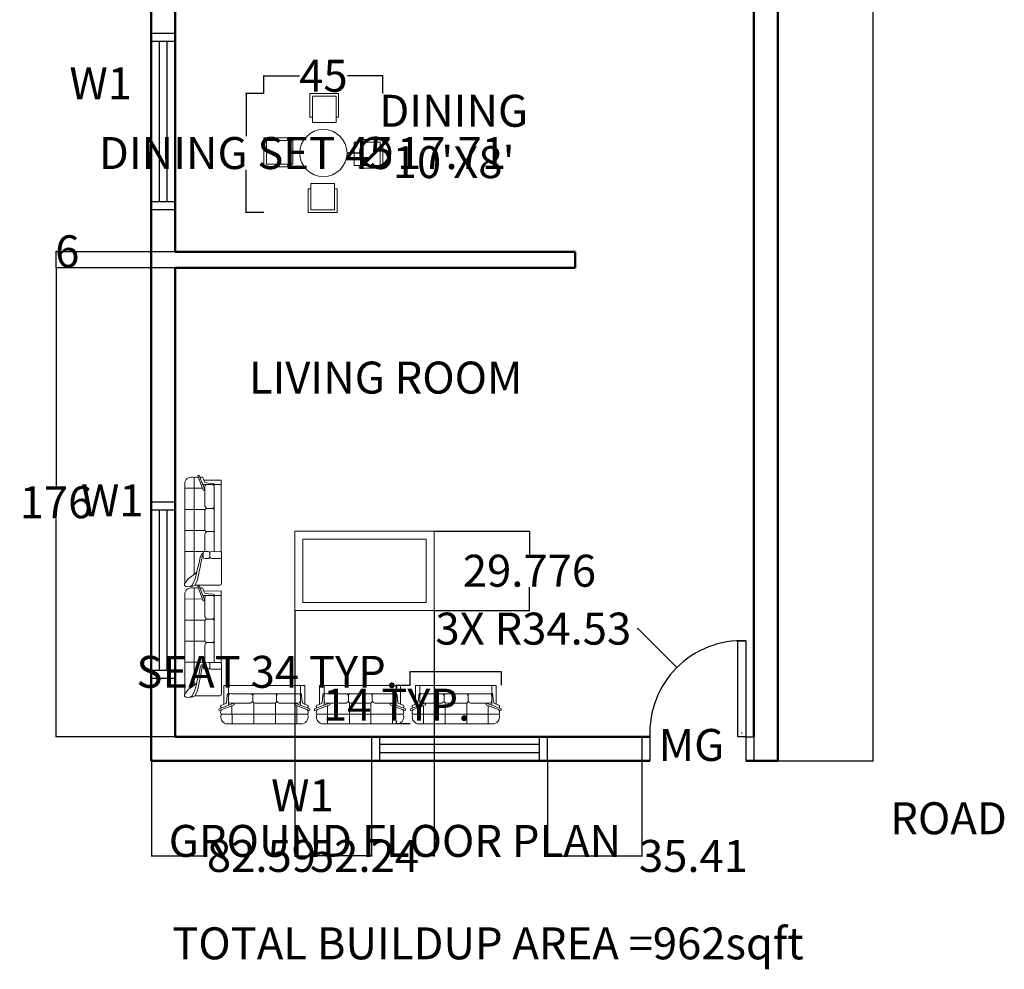
# Model space of a CAD drawing. Units: inches. Extents: x -15 to 810, y -55 to 662.
# Tile 1 of 3: x -7 to 362, y -55 to 302. Entities that reach past the tile are written whole.
import ezdxf
from ezdxf.enums import TextEntityAlignment as Align

# ---------------------------------------------------------------- set-up
doc = ezdxf.new("R2010")
doc.units = ezdxf.units.IN
doc.header["$MEASUREMENT"] = 0
for name, color, linetype, lineweight in [('A-ANNO-DIMS', 2, 'Continuous', 18), ('A-ANNO-TEXT', 1, 'Continuous', 25), ('A-AREA-IDEN', 1, 'Continuous', 25), ('A-DOOR', 2, 'Continuous', 25), ('A-FURN', 8, 'Continuous', 18), ('A-GLAZ', 4, 'Continuous', 18), ('A-WALL', 6, 'Continuous', 50)]:
    doc.layers.add(name, color=color, linetype=linetype, lineweight=lineweight)
doc.layers.add('Layer3', color=4, linetype='Continuous')
doc.styles.get("Standard").update_dxf_attribs({"font": 'arial.ttf'})
doc.dimstyles.get("Standard").update_dxf_attribs({"dimtxt": 12, "dimasz": 0.18, "dimexe": 0.18, "dimexo": 0.0625, "dimgap": 0.09, "dimtad": 0, "dimtih": 1, "dimtoh": 1, "dimdec": 0, "dimzin": 0, "dimdsep": 46, "dimlunit": 4, "dimtxsty": 'Standard', "dimcen": 0.09, "dimadec": 0, "dimazin": 0, "dimtfac": 1, "dimtdec": 0, "dimtofl": 0, "dimtmove": 0, "dimatfit": 3, "dimfxl": 1, "dimtolj": 1, "dimtzin": 0, "dimarcsym": 0})

# ---------------------------------------------------------------- blocks, each defined once
blk = doc.blocks.new('A$C21DD57CF')
for p, q in [((0, 682), (8, 763)), ((0, 682), (8, 763)), ((37, 628), (0, 682)), ((37, 628), (0, 682)), ((8, 763), (29, 794)), ((8, 763), (29, 794)), ((16, 616), (16, 655)), ((16, 616), (16, 655)), ((29, 794), (63, 792)), ((29, 794), (63, 792)), ((63, 792), (74, 786)), ((63, 792), (74, 786)), ((74, 786), (2250, 786)), ((74, 786), (173, 714)), ((74, 786), (2250, 786)), ((74, 786), (173, 714)), ((173, 714), (247, 611)), ((173, 714), (247, 611)), ((640, 786), (761, 786)), ((640, 786), (761, 786)), ((761, 786), (761, 356)), ((761, 786), (761, 356)), ((1211, 356), (1211, 786)), ((1211, 786), (1661, 786)), ((1211, 356), (1211, 786)), ((1211, 786), (1661, 786)), ((1661, 786), (1661, 347)), ((1661, 786), (1661, 347)), ((2116, 783), (2119, 410)), ((2116, 783), (2119, 410)), ((35, 572), (16, 616)), ((35, 572), (16, 616)), ((35, 574), (141, 516)), ((35, 574), (141, 516)), ((36, 32), (36, 574)), ((36, 32), (36, 574)), ((159, 572), (37, 631)), ((159, 572), (37, 631)), ((141, 516), (218, 501)), ((141, 516), (218, 501)), ((228, 550), (159, 572)), ((228, 550), (159, 572)), ((218, 501), (326, 479)), ((218, 501), (326, 479)), ((334, 528), (228, 550)), ((334, 528), (228, 550)), ((247, 611), (314, 530)), ((247, 611), (314, 530)), ((274, 586), (2345, 589)), ((274, 586), (2345, 589)), ((326, 479), (422, 460)), ((326, 479), (422, 460)), ((414, 506), (334, 528)), ((414, 506), (334, 528)), ((517, 484), (414, 506)), ((517, 484), (414, 506)), ((422, 460), (501, 445)), ((422, 460), (501, 445)), ((501, 445), (660, 413)), ((501, 445), (660, 413)), ((636, 460), (517, 484)), ((636, 460), (517, 484)), ((703, 430), (636, 460)), ((703, 430), (636, 460)), ((701, 430), (719, 398)), ((701, 430), (719, 398)), ((703, 427), (703, 430)), ((703, 427), (703, 430)), ((2346, 495), (2076, 394)), ((2346, 495), (2076, 394)), ((2082, 357), (2343, 458)), ((2082, 357), (2343, 458)), ((2343, 458), (2393, 477)), ((2343, 458), (2393, 477)), ((2356, 445), (2343, 458)), ((2356, 445), (2343, 458)), ((2346, 495), (2346, 509)), ((2346, 495), (2346, 509)), ((2346, 495), (2386, 508)), ((2346, 495), (2386, 508)), ((2356, 428), (2354, 413)), ((2356, 428), (2354, 413)), ((2356, 428), (2356, 445)), ((2356, 428), (2356, 445)), ((2394, 499), (2386, 508)), ((2394, 499), (2386, 508)), ((2393, 477), (2397, 489)), ((2393, 477), (2397, 489)), ((2397, 489), (2394, 499)), ((2397, 489), (2394, 499)), ((36, 32), (36, 400)), ((36, 32), (36, 400)), ((605, 205), (613, 235)), ((605, 205), (613, 235)), ((617, 384), (606, 354)), ((617, 384), (606, 354)), ((606, 294), (606, 354)), ((606, 294), (606, 354)), ((606, 294), (609, 276)), ((606, 294), (609, 276)), ((609, 276), (619, 264)), ((609, 276), (619, 264)), ((613, 235), (619, 244)), ((613, 235), (619, 244)), ((646, 398), (617, 384)), ((646, 398), (617, 384)), ((619, 264), (644, 249)), ((619, 264), (644, 249)), ((619, 244), (640, 249)), ((619, 244), (640, 249)), ((736, 250), (642, 250)), ((736, 250), (642, 250)), ((719, 398), (646, 398)), ((719, 398), (646, 398)), ((660, 413), (685, 398)), ((660, 413), (685, 398)), ((719, 398), (731, 398)), ((719, 398), (731, 398)), ((731, 398), (748, 389)), ((731, 398), (748, 389)), ((733, 249), (748, 244)), ((733, 249), (748, 244)), ((735, 249), (752, 264)), ((735, 249), (752, 264)), ((748, 389), (757, 371)), ((748, 389), (757, 371)), ((748, 244), (754, 233)), ((748, 244), (754, 233)), ((752, 264), (756, 287)), ((752, 264), (756, 287)), ((754, 233), (756, 24)), ((754, 233), (756, 24)), ((757, 371), (756, 287)), ((757, 371), (756, 287)), ((761, 356), (1134, 356)), ((761, 356), (1134, 356)), ((797, 356), (1134, 356)), ((797, 356), (1134, 356)), ((1134, 356), (1160, 345)), ((1134, 356), (1160, 345)), ((1160, 345), (1180, 324)), ((1160, 345), (1180, 324)), ((1180, 324), (1186, 313)), ((1180, 324), (1186, 313)), ((1185, 192), (1185, 315)), ((1185, 192), (1185, 315)), ((1225, 356), (1633, 356)), ((1225, 356), (1633, 356)), ((1633, 356), (1667, 345)), ((1633, 356), (1667, 345)), ((1667, 345), (1685, 326)), ((1667, 345), (1685, 326)), ((1684, 324), (1705, 338)), ((1684, 324), (1705, 338)), ((1685, 326), (1685, 159)), ((1685, 326), (1685, 159)), ((1705, 338), (1733, 356)), ((1705, 338), (1733, 356)), ((1733, 356), (2144, 356)), ((1733, 356), (2111, 356)), ((1733, 356), (2144, 356)), ((1733, 356), (2111, 356)), ((2076, 394), (2074, 374)), ((2076, 394), (2074, 374)), ((2074, 374), (2078, 364)), ((2074, 374), (2078, 364)), ((2078, 364), (2082, 357)), ((2078, 364), (2082, 357)), ((2119, 356), (2119, 371)), ((2119, 356), (2119, 371)), ((2144, 356), (2178, 351)), ((2144, 356), (2178, 351)), ((2178, 351), (2192, 333)), ((2178, 351), (2192, 333)), ((2192, 333), (2194, 320)), ((2192, 333), (2194, 320)), ((2194, 348), (2193, 348)), ((2194, 348), (2193, 348)), ((2194, 400), (2194, 5)), ((2194, 400), (2194, 5)), ((2225, 287), (2218, 183)), ((2225, 287), (2218, 183)), ((2242, 360), (2225, 287)), ((2242, 360), (2225, 287)), ((2286, 378), (2242, 360)), ((2286, 378), (2242, 360)), ((2346, 403), (2288, 378)), ((2346, 403), (2288, 378)), ((2288, 378), (2289, 5)), ((2288, 378), (2289, 5)), ((2354, 413), (2346, 403)), ((2354, 413), (2346, 403)), ((35, 34), (51, 7)), ((35, 34), (51, 7)), ((51, 7), (84, 0)), ((51, 7), (84, 0)), ((732, 0), (83, 0)), ((732, 0), (83, 0)), ((605, 27), (615, 10)), ((605, 27), (615, 10)), ((606, 25), (606, 208)), ((606, 25), (606, 208)), ((732, 0), (606, 0)), ((732, 0), (606, 0)), ((615, 10), (636, 0)), ((615, 10), (636, 0)), ((731, 0), (748, 10)), ((731, 0), (748, 10)), ((740, 5), (2289, 5)), ((740, 5), (2289, 5)), ((748, 10), (756, 27)), ((748, 10), (756, 27)), ((2131, 156), (752, 156)), ((2131, 156), (752, 156)), ((1152, 156), (1171, 160)), ((1152, 156), (1171, 160)), ((1171, 160), (1183, 174)), ((1171, 160), (1183, 174)), ((1183, 174), (1185, 192)), ((1183, 174), (1185, 192)), ((1185, 192), (1200, 160)), ((1185, 192), (1200, 160)), ((1200, 160), (1232, 156)), ((1200, 160), (1232, 156)), ((1676, 174), (1649, 154)), ((1676, 174), (1649, 154)), ((1687, 195), (1676, 174)), ((1687, 195), (1676, 174)), ((1684, 195), (1705, 164)), ((1684, 195), (1705, 164)), ((1705, 164), (1736, 154)), ((1705, 164), (1736, 154)), ((2170, 161), (2131, 156)), ((2170, 161), (2131, 156)), ((2191, 178), (2170, 161)), ((2191, 178), (2170, 161)), ((2194, 194), (2191, 178)), ((2194, 194), (2191, 178)), ((2210, 156), (2194, 156)), ((2210, 156), (2194, 156)), ((2218, 183), (2210, 156)), ((2218, 183), (2210, 156))]:
    blk.add_line(p, q)
for centre, radius, start, end in [((2206, 643), 150, 338.8976, 73.2177), ((2206, 643), 150, 338.8976, 73.2177), ((2286, 548), 72.2, 326.352, 34.4802), ((2286, 548), 72.2, 326.352, 34.4802), ((1228, 313), 43.2, 92.4362, 179.0526), ((1228, 313), 43.2, 92.4362, 179.0526)]:
    blk.add_arc(centre, radius, start, end)
blk = doc.blocks.new('A$C05430CFC')
for p, q in [((155, 802, -343), (1764, 802, -343)), ((155, 802, -343), (1764, 802, -343)), ((276, 802, -343), (276, 424, -343)), ((276, 802, -343), (276, 424, -343)), ((726, 372, -343), (726, 802, -343)), ((726, 802, -343), (1176, 802, -343)), ((726, 372, -343), (726, 802, -343)), ((726, 802, -343), (1176, 802, -343)), ((1176, 802, -343), (1176, 362, -343)), ((1176, 802, -343), (1176, 362, -343)), ((1635, 802, -343), (1636, 426, -343)), ((1635, 802, -343), (1636, 426, -343)), ((0, 501, -343), (2, 511, -343)), ((0, 501, -343), (2, 511, -343)), ((4, 489, -343), (0, 501, -343)), ((4, 489, -343), (0, 501, -343)), ((2, 511, -343), (10, 521, -343)), ((2, 511, -343), (10, 521, -343)), ((315, 371, -343), (4, 489, -343)), ((315, 371, -343), (4, 489, -343)), ((14, 521, -343), (321, 407, -343)), ((14, 521, -343), (321, 407, -343)), ((39, 444, -343), (41, 418, -343)), ((39, 444, -343), (41, 418, -343)), ((40, 458, -343), (50, 468, -343)), ((40, 458, -343), (50, 468, -343)), ((40, 441, -343), (40, 458, -343)), ((40, 441, -343), (40, 458, -343)), ((41, 418, -343), (56, 411, -343)), ((41, 418, -343), (56, 411, -343)), ((50, 419, -343), (51, 419, -343)), ((50, 419, -343), (51, 419, -343)), ((51, 602, -343), (1862, 602, -343)), ((51, 602, -343), (1862, 602, -343)), ((51, 502, -343), (51, 522, -343)), ((51, 502, -343), (51, 522, -343)), ((51, 502, -343), (66, 502, -343)), ((51, 502, -343), (66, 502, -343)), ((51, 416, -343), (110, 391, -343)), ((51, 416, -343), (110, 391, -343)), ((201, 2, -343), (201, 414, -343)), ((201, 2, -343), (201, 414, -343)), ((1900, 525, -343), (1591, 409, -343)), ((1900, 525, -343), (1591, 409, -343)), ((1597, 372, -343), (1907, 492, -343)), ((1597, 372, -343), (1907, 492, -343)), ((1710, 416, -343), (1710, 2, -343)), ((1710, 416, -343), (1710, 2, -343)), ((1861, 419, -343), (1801, 393, -343)), ((1861, 419, -343), (1801, 393, -343)), ((1871, 421, -343), (1855, 414, -343)), ((1871, 421, -343), (1855, 414, -343)), ((1860, 510, -343), (1860, 524, -343)), ((1860, 510, -343), (1860, 524, -343)), ((1871, 460, -343), (1861, 470, -343)), ((1871, 460, -343), (1861, 470, -343)), ((1861, 422, -343), (1861, 421, -343)), ((1861, 422, -343), (1861, 421, -343)), ((1871, 443, -343), (1871, 460, -343)), ((1871, 443, -343), (1871, 460, -343)), ((1873, 446, -343), (1871, 421, -343)), ((1873, 446, -343), (1871, 421, -343)), ((1909, 514, -343), (1900, 525, -343)), ((1909, 514, -343), (1900, 525, -343)), ((1907, 492, -343), (1911, 504, -343)), ((1907, 492, -343), (1911, 504, -343)), ((1911, 504, -343), (1909, 514, -343)), ((1911, 504, -343), (1909, 514, -343)), ((109, 397, -343), (109, 0, -343)), ((109, 397, -343), (109, 0, -343)), ((110, 391, -343), (159, 372, -343)), ((110, 391, -343), (159, 372, -343)), ((153, 380, -343), (172, 300, -343)), ((153, 380, -343), (172, 300, -343)), ((172, 300, -343), (180, 196, -343)), ((172, 300, -343), (180, 196, -343)), ((205, 346, -343), (200, 312, -343)), ((205, 346, -343), (200, 312, -343)), ((200, 232, -343), (206, 191, -343)), ((200, 232, -343), (206, 191, -343)), ((201, 366, -343), (202, 366, -343)), ((201, 366, -343), (202, 366, -343)), ((219, 364, -343), (205, 346, -343)), ((219, 364, -343), (205, 346, -343)), ((259, 371, -343), (219, 364, -343)), ((259, 371, -343), (219, 364, -343)), ((257, 370, -343), (278, 371, -343)), ((257, 370, -343), (278, 371, -343)), ((276, 372, -343), (648, 372, -343)), ((276, 372, -343), (648, 372, -343)), ((312, 372, -343), (648, 372, -343)), ((312, 372, -343), (648, 372, -343)), ((319, 378, -343), (315, 371, -343)), ((319, 378, -343), (315, 371, -343)), ((323, 388, -343), (319, 378, -343)), ((323, 388, -343), (319, 378, -343)), ((321, 407, -343), (323, 388, -343)), ((321, 407, -343), (323, 388, -343)), ((648, 372, -343), (675, 360, -343)), ((648, 372, -343), (675, 360, -343)), ((675, 360, -343), (695, 339, -343)), ((675, 360, -343), (695, 339, -343)), ((695, 339, -343), (701, 329, -343)), ((695, 339, -343), (701, 329, -343)), ((698, 190, -343), (698, 214, -343)), ((698, 190, -343), (698, 214, -343)), ((698, 207, -343), (715, 176, -343)), ((698, 207, -343), (715, 176, -343)), ((700, 255, -343), (700, 330, -343)), ((700, 175, -343), (700, 330, -343)), ((700, 255, -343), (700, 330, -343)), ((700, 175, -343), (700, 330, -343)), ((740, 372, -343), (1147, 372, -343)), ((740, 372, -343), (1147, 372, -343)), ((1147, 372, -343), (1182, 360, -343)), ((1147, 372, -343), (1182, 360, -343)), ((1182, 360, -343), (1200, 342, -343)), ((1182, 360, -343), (1200, 342, -343)), ((1202, 210, -343), (1190, 190, -343)), ((1202, 210, -343), (1190, 190, -343)), ((1199, 339, -343), (1219, 353, -343)), ((1199, 339, -343), (1219, 353, -343)), ((1199, 210, -343), (1219, 179, -343)), ((1199, 210, -343), (1219, 179, -343)), ((1200, 342, -343), (1200, 175, -343)), ((1200, 342, -343), (1200, 175, -343)), ((1219, 353, -343), (1247, 372, -343)), ((1219, 353, -343), (1247, 372, -343)), ((1247, 372, -343), (1626, 372, -343)), ((1247, 372, -343), (1659, 372, -343)), ((1247, 372, -343), (1626, 372, -343)), ((1247, 372, -343), (1659, 372, -343)), ((1591, 409, -343), (1589, 389, -343)), ((1591, 409, -343), (1589, 389, -343)), ((1589, 389, -343), (1593, 380, -343)), ((1589, 389, -343), (1593, 380, -343)), ((1593, 380, -343), (1597, 372, -343)), ((1593, 380, -343), (1597, 372, -343)), ((1633, 372, -343), (1633, 387, -343)), ((1633, 372, -343), (1633, 387, -343)), ((1659, 372, -343), (1692, 366, -343)), ((1659, 372, -343), (1692, 366, -343)), ((1692, 366, -343), (1706, 348, -343)), ((1692, 366, -343), (1706, 348, -343)), ((1711, 229, -343), (1705, 188, -343)), ((1711, 229, -343), (1705, 188, -343)), ((1706, 348, -343), (1710, 324, -343)), ((1706, 348, -343), (1710, 324, -343)), ((1712, 234, -343), (1706, 193, -343)), ((1712, 234, -343), (1706, 193, -343)), ((1740, 303, -343), (1733, 198, -343)), ((1740, 303, -343), (1733, 198, -343)), ((1757, 376, -343), (1740, 303, -343)), ((1757, 376, -343), (1740, 303, -343)), ((1801, 393, -343), (1757, 376, -343)), ((1801, 393, -343), (1757, 376, -343)), ((1803, 394, -343), (1804, 2, -343)), ((1803, 394, -343), (1804, 2, -343)), ((1804, 2, -343), (109, 2, -343)), ((109, 2, -343), (201, 2, -343)), ((1804, 2, -343), (109, 2, -343)), ((109, 2, -343), (201, 2, -343)), ((180, 196, -343), (188, 170, -343)), ((180, 196, -343), (188, 170, -343)), ((188, 170, -343), (204, 170, -343)), ((188, 170, -343), (204, 170, -343)), ((206, 191, -343), (227, 174, -343)), ((206, 191, -343), (227, 174, -343)), ((227, 174, -343), (270, 172, -343)), ((227, 174, -343), (270, 172, -343)), ((1646, 172, -343), (267, 172, -343)), ((1646, 172, -343), (267, 172, -343)), ((651, 169, -343), (686, 176, -343)), ((651, 169, -343), (686, 176, -343)), ((686, 176, -343), (698, 190, -343)), ((686, 176, -343), (698, 190, -343)), ((715, 176, -343), (747, 172, -343)), ((715, 176, -343), (747, 172, -343)), ((1190, 190, -343), (1164, 169, -343)), ((1190, 190, -343), (1164, 169, -343)), ((1219, 179, -343), (1251, 169, -343)), ((1219, 179, -343), (1251, 169, -343)), ((1684, 171, -343), (1646, 172, -343)), ((1684, 171, -343), (1646, 172, -343)), ((1705, 188, -343), (1684, 171, -343)), ((1705, 188, -343), (1684, 171, -343)), ((1725, 172, -343), (1708, 172, -343)), ((1725, 172, -343), (1708, 172, -343)), ((1733, 198, -343), (1725, 172, -343)), ((1733, 198, -343), (1725, 172, -343))]:
    blk.add_line(p, q)
for centre, radius, start, end in [((190, 656, -343), 150, 103.5221, 201.2641), ((190, 656, -343), 150, 103.5221, 201.2641), ((1720, 658, -343), 150, 338.8976, 73.2177), ((1720, 658, -343), 150, 338.8976, 73.2177), ((110, 561, -343), 72.2, 145.6816, 213.8098), ((110, 561, -343), 72.2, 145.6816, 213.8098), ((1801, 563, -343), 72.2, 326.352, 34.4802), ((1801, 563, -343), 72.2, 326.352, 34.4802), ((743, 329, -343), 43.2, 92.4362, 179.0526), ((743, 329, -343), 43.2, 92.4362, 179.0526)]:
    blk.add_arc(centre, radius, start, end)
blk = doc.blocks.new('A$C791C5AB8')
for p, q in [((0.873, 1.816), (0.873, 2.266)), ((0.873, 2.266), (1.423, 2.266)), ((1.423, 2.266), (1.423, 1.816)), ((0.923, 2.216), (0.923, 1.716)), ((1.373, 2.216), (0.923, 2.216)), ((1.373, 1.716), (1.373, 2.216)), ((0.923, 1.816), (0.873, 1.816)), ((1.373, 1.716), (0.923, 1.716)), ((1.423, 1.816), (1.373, 1.816)), ((0, 0.873), (0, 1.423)), ((0, 1.423), (0.45, 1.423)), ((0.05, 1.373), (0.05, 0.923)), ((0.55, 1.373), (0.05, 1.373)), ((0.45, 1.423), (0.45, 1.373)), ((0.55, 1.373), (0.55, 0.923)), ((1.716, 0.893), (1.716, 1.343)), ((2.216, 1.343), (1.716, 1.343)), ((1.816, 1.343), (1.816, 1.393)), ((1.816, 1.393), (2.266, 1.393)), ((2.216, 0.893), (2.216, 1.343)), ((2.266, 1.393), (2.266, 0.843)), ((0.45, 0.873), (0, 0.873)), ((0.05, 0.923), (0.55, 0.923)), ((0.45, 0.923), (0.45, 0.873)), ((1.716, 0.893), (2.216, 0.893)), ((1.816, 0.843), (1.816, 0.893)), ((2.266, 0.843), (1.816, 0.843)), ((0.843, 0), (0.843, 0.45)), ((0.843, 0.45), (0.893, 0.45)), ((0.893, 0.55), (0.893, 0.05)), ((0.893, 0.55), (1.343, 0.55)), ((1.343, 0.05), (1.343, 0.55)), ((1.343, 0.45), (1.393, 0.45)), ((1.393, 0.45), (1.393, 0)), ((1.393, 0), (0.843, 0)), ((0.893, 0.05), (1.343, 0.05))]:
    blk.add_line(p, q)
blk.add_circle((1.133, 1.133), 0.45)
blk = doc.blocks.new('gh')
at = {"layer": 'Layer3'}
for p, q in [((0, 0), (0, -9)), ((63, 0), (3, 0)), ((3, 0), (3, -9)), ((63, -9), (63, 0)), ((66, -9), (66, 0)), ((63, -3), (3, -3)), ((3, -6), (63, -6)), ((3, -9), (63, -9))]:
    blk.add_line(p, q, dxfattribs=at)
blk = doc.blocks.new('*D22')
at = {"layer": 'A-ANNO-DIMS', "color": 0, "lineweight": -2, "transparency": 16777216}
for p, q in [((139.31, 57.06), (139.13, 57.06)), ((139.31, 51.99), (139.31, 57.24)), ((173.33, 57.06), (139.49, 57.06)), ((173.51, 51.99), (173.51, 57.24))]:
    blk.add_line(p, q, dxfattribs=at)
at = {"layer": 'A-ANNO-DIMS', "color": 0, "transparency": 16777216}
for points in [[(139.49, 57.09), (139.49, 57.03), (139.31, 57.06)], [(173.33, 57.09), (173.33, 57.03), (173.51, 57.06)]]:
    blk.add_solid(points, dxfattribs=at)
at = {"layer": 'Defpoints', "color": 0, "transparency": 16777216}
for p in [(139.31, 57.06), (139.31, 51.93), (173.51, 51.93)]:
    blk.add_point(p, dxfattribs=at)
at = {"layer": 'A-ANNO-DIMS', "color": 0, "transparency": 16777216, "insert": (85.64, 57.06), "char_height": 12, "attachment_point": 5}
blk.add_mtext('\\A1;SEAT 34 TYP.', dxfattribs=at)
blk = doc.blocks.new('*D23')
at = {"layer": 'A-ANNO-DIMS', "color": 0, "lineweight": -2, "transparency": 16777216}
for p, q in [((139.25, 51.93), (134, 51.93)), ((134.18, 51.75), (134.18, 50.87)), ((139.25, 37.58), (134, 37.58)), ((134.18, 37.76), (134.18, 38.64))]:
    blk.add_line(p, q, dxfattribs=at)
at = {"layer": 'A-ANNO-DIMS', "color": 0, "transparency": 16777216}
for points in [[(134.15, 51.75), (134.21, 51.75), (134.18, 51.93)], [(134.15, 37.76), (134.21, 37.76), (134.18, 37.58)]]:
    blk.add_solid(points, dxfattribs=at)
at = {"layer": 'Defpoints', "color": 0, "transparency": 16777216}
for p in [(139.31, 51.93), (134.18, 37.58), (139.31, 37.58)]:
    blk.add_point(p, dxfattribs=at)
at = {"layer": 'A-ANNO-DIMS', "color": 0, "transparency": 16777216, "insert": (134.18, 44.75), "char_height": 12, "attachment_point": 5}
blk.add_mtext('\\A1;14 TYP.', dxfattribs=at)
blk = doc.blocks.new('*D28')
at = {"layer": 'A-ANNO-DIMS', "color": 0, "lineweight": -2, "transparency": 16777216}
for p, q in [((84.38, 274.06), (77.57, 274.06)), ((77.75, 273.88), (77.75, 258.06)), ((77.75, 229.65), (77.75, 245.47)), ((84.38, 229.47), (77.57, 229.47))]:
    blk.add_line(p, q, dxfattribs=at)
at = {"layer": 'A-ANNO-DIMS', "color": 0, "transparency": 16777216}
for points in [[(77.72, 273.88), (77.78, 273.88), (77.75, 274.06)], [(77.72, 229.65), (77.78, 229.65), (77.75, 229.47)]]:
    blk.add_solid(points, dxfattribs=at)
at = {"layer": 'Defpoints', "color": 0, "transparency": 16777216}
for p in [(77.75, 274.06), (84.44, 274.06), (84.44, 229.47)]:
    blk.add_point(p, dxfattribs=at)
at = {"layer": 'A-ANNO-DIMS', "color": 0, "transparency": 16777216, "insert": (77.75, 251.76), "char_height": 12, "attachment_point": 5}
blk.add_mtext('\\A1;DINING SET 45', dxfattribs=at)
blk = doc.blocks.new('*D29')
at = {"layer": 'A-ANNO-DIMS', "color": 0, "lineweight": -2, "transparency": 16777216}
for p, q in [((84.44, 274.12), (84.44, 280.93)), ((84.62, 280.75), (97.77, 280.75)), ((128.85, 280.75), (115.71, 280.75)), ((129.03, 274.12), (129.03, 280.93))]:
    blk.add_line(p, q, dxfattribs=at)
at = {"layer": 'A-ANNO-DIMS', "color": 0, "transparency": 16777216}
for points in [[(84.62, 280.78), (84.62, 280.72), (84.44, 280.75)], [(128.85, 280.78), (128.85, 280.72), (129.03, 280.75)]]:
    blk.add_solid(points, dxfattribs=at)
at = {"layer": 'Defpoints', "color": 0, "transparency": 16777216}
for p in [(129.03, 280.75), (84.44, 274.06), (129.03, 274.06)]:
    blk.add_point(p, dxfattribs=at)
at = {"layer": 'A-ANNO-DIMS', "color": 0, "transparency": 16777216, "insert": (106.74, 280.75), "char_height": 12, "attachment_point": 5}
blk.add_mtext('\\A1;45', dxfattribs=at)
blk = doc.blocks.new('*D35')
at = {"layer": 'A-ANNO-DIMS', "color": 0, "lineweight": -2, "transparency": 16777216}
for p, q in [((277.25, 613.7), (313.12, 613.7)), ((312.94, 613.52), (312.94, 324.92)), ((312.94, 23.88), (312.94, 312.49)), ((277.25, 23.7), (313.12, 23.7))]:
    blk.add_line(p, q, dxfattribs=at)
at = {"layer": 'A-ANNO-DIMS', "color": 0, "transparency": 16777216}
for points in [[(312.91, 613.52), (312.97, 613.52), (312.94, 613.7)], [(312.91, 23.88), (312.97, 23.88), (312.94, 23.7)]]:
    blk.add_solid(points, dxfattribs=at)
at = {"layer": 'Defpoints', "color": 0, "transparency": 16777216}
for p in [(277.19, 613.7), (312.94, 613.7), (277.19, 23.7)]:
    blk.add_point(p, dxfattribs=at)
at = {"layer": 'A-ANNO-DIMS', "color": 0, "transparency": 16777216, "insert": (312.94, 318.7), "char_height": 12, "attachment_point": 5}
blk.add_mtext('\\A1;590', dxfattribs=at)
blk = doc.blocks.new('*D38')
at = {"layer": 'A-ANNO-DIMS', "color": 0, "lineweight": -2, "transparency": 16777216}
for p, q in [((51.12, 208.7), (6.26, 208.7)), ((6.44, 208.52), (6.44, 126.92)), ((6.44, 32.88), (6.44, 114.49)), ((51.12, 32.7), (6.26, 32.7))]:
    blk.add_line(p, q, dxfattribs=at)
at = {"layer": 'A-ANNO-DIMS', "color": 0, "transparency": 16777216}
for points in [[(6.41, 208.52), (6.47, 208.52), (6.44, 208.7)], [(6.41, 32.88), (6.47, 32.88), (6.44, 32.7)]]:
    blk.add_solid(points, dxfattribs=at)
at = {"layer": 'Defpoints', "color": 0, "transparency": 16777216}
for p in [(6.44, 208.7), (51.19, 208.7), (51.19, 32.7)]:
    blk.add_point(p, dxfattribs=at)
at = {"layer": 'A-ANNO-DIMS', "color": 0, "transparency": 16777216, "insert": (6.44, 120.7), "char_height": 12, "attachment_point": 5}
blk.add_mtext('\\A1;176', dxfattribs=at)
blk = doc.blocks.new('*D39')
at = {"layer": 'A-ANNO-DIMS', "color": 0, "lineweight": -2, "transparency": 16777216}
for p, q in [((51.12, 214.7), (6.26, 214.7)), ((6.44, 214.7), (6.44, 214.88)), ((6.44, 214.88), (6.62, 214.88)), ((6.44, 208.88), (6.44, 214.52)), ((51.12, 208.7), (6.26, 208.7))]:
    blk.add_line(p, q, dxfattribs=at)
at = {"layer": 'A-ANNO-DIMS', "color": 0, "transparency": 16777216}
for points in [[(6.41, 214.52), (6.47, 214.52), (6.44, 214.7)], [(6.41, 208.88), (6.47, 208.88), (6.44, 208.7)]]:
    blk.add_solid(points, dxfattribs=at)
at = {"layer": 'Defpoints', "color": 0, "transparency": 16777216}
for p in [(6.44, 214.7), (51.19, 214.7), (51.19, 208.7)]:
    blk.add_point(p, dxfattribs=at)
at = {"layer": 'A-ANNO-DIMS', "color": 0, "transparency": 16777216, "insert": (10.67, 214.88), "char_height": 12, "attachment_point": 5}
blk.add_mtext('\\A1;6', dxfattribs=at)
blk = doc.blocks.new('*D40')
at = {"layer": 'A-ANNO-DIMS', "color": 0, "lineweight": -2, "transparency": 16777216}
for p, q in [((42.19, 23.64), (42.19, -12.23)), ((124.78, 23.74), (124.78, -12.23)), ((42.37, -12.05), (63.12, -12.05)), ((124.6, -12.05), (103.84, -12.05))]:
    blk.add_line(p, q, dxfattribs=at)
at = {"layer": 'A-ANNO-DIMS', "color": 0, "transparency": 16777216}
for points in [[(42.37, -12.02), (42.37, -12.08), (42.19, -12.05)], [(124.6, -12.02), (124.6, -12.08), (124.78, -12.05)]]:
    blk.add_solid(points, dxfattribs=at)
at = {"layer": 'Defpoints', "color": 0, "transparency": 16777216}
for p in [(42.19, 23.7), (124.78, 23.8), (124.78, -12.05)]:
    blk.add_point(p, dxfattribs=at)
at = {"layer": 'A-ANNO-DIMS', "color": 0, "transparency": 16777216, "insert": (83.48, -12.05), "char_height": 12, "attachment_point": 5}
blk.add_mtext('\\A1;82.59', dxfattribs=at)
blk = doc.blocks.new('*D41')
at = {"layer": 'A-ANNO-DIMS', "color": 0, "lineweight": -2, "transparency": 16777216}
for p, q in [((190.78, 23.74), (190.78, -12.23)), ((226.19, 23.64), (226.19, -12.23)), ((190.96, -12.05), (226.01, -12.05)), ((226.19, -12.05), (226.37, -12.05))]:
    blk.add_line(p, q, dxfattribs=at)
at = {"layer": 'A-ANNO-DIMS', "color": 0, "transparency": 16777216}
for points in [[(190.96, -12.02), (190.96, -12.08), (190.78, -12.05)], [(226.01, -12.02), (226.01, -12.08), (226.19, -12.05)]]:
    blk.add_solid(points, dxfattribs=at)
at = {"layer": 'Defpoints', "color": 0, "transparency": 16777216}
for p in [(190.78, 23.8), (226.19, 23.7), (226.19, -12.05)]:
    blk.add_point(p, dxfattribs=at)
at = {"layer": 'A-ANNO-DIMS', "color": 0, "transparency": 16777216, "insert": (245.54, -12.05), "char_height": 12, "attachment_point": 5}
blk.add_mtext('\\A1;35.41', dxfattribs=at)
blk = doc.blocks.new('*D51')
at = {"layer": 'A-ANNO-DIMS', "color": 0, "lineweight": -2, "transparency": 16777216}
for p, q in [((96.03, 80.06), (96.03, -12.23)), ((148.27, 80.06), (148.27, -12.23)), ((96.21, -12.05), (101.84, -12.05)), ((148.09, -12.05), (142.46, -12.05))]:
    blk.add_line(p, q, dxfattribs=at)
at = {"layer": 'A-ANNO-DIMS', "color": 0, "transparency": 16777216}
for points in [[(96.21, -12.02), (96.21, -12.08), (96.03, -12.05)], [(148.09, -12.02), (148.09, -12.08), (148.27, -12.05)]]:
    blk.add_solid(points, dxfattribs=at)
at = {"layer": 'Defpoints', "color": 0, "transparency": 16777216}
for p in [(96.03, 80.12), (148.27, 80.12), (148.27, -12.05)]:
    blk.add_point(p, dxfattribs=at)
at = {"layer": 'A-ANNO-DIMS', "color": 0, "transparency": 16777216, "insert": (122.15, -12.05), "char_height": 12, "attachment_point": 5}
blk.add_mtext('\\A1;52.24', dxfattribs=at)
blk = doc.blocks.new('*D52')
at = {"layer": 'A-ANNO-DIMS', "color": 0, "lineweight": -2, "transparency": 16777216}
for p, q in [((148.33, 109.89), (184.2, 109.89)), ((184.02, 109.71), (184.02, 101.22)), ((184.02, 80.3), (184.02, 88.79)), ((148.33, 80.12), (184.2, 80.12))]:
    blk.add_line(p, q, dxfattribs=at)
at = {"layer": 'A-ANNO-DIMS', "color": 0, "transparency": 16777216}
for points in [[(183.99, 109.71), (184.05, 109.71), (184.02, 109.89)], [(183.99, 80.3), (184.05, 80.3), (184.02, 80.12)]]:
    blk.add_solid(points, dxfattribs=at)
at = {"layer": 'Defpoints', "color": 0, "transparency": 16777216}
for p in [(148.27, 109.89), (148.27, 80.12), (184.02, 80.12)]:
    blk.add_point(p, dxfattribs=at)
at = {"layer": 'A-ANNO-DIMS', "color": 0, "transparency": 16777216, "insert": (184.02, 95.01), "char_height": 12, "attachment_point": 5}
blk.add_mtext('\\A1;29.776', dxfattribs=at)
blk = doc.blocks.new('*D56')
at = {"layer": 'A-ANNO-DIMS', "color": 0, "lineweight": -2, "transparency": 16777216}
for p, q in [((224.44, 73.27), (224.62, 73.27)), ((224.62, 73.27), (239.14, 58.75)), ((263.6, 34.2), (263.78, 34.2)), ((263.69, 34.11), (263.69, 34.29))]:
    blk.add_line(p, q, dxfattribs=at)
at = {"layer": 'A-ANNO-DIMS', "color": 0, "transparency": 16777216}
blk.add_solid([(239.16, 58.77), (239.12, 58.73), (239.27, 58.62)], dxfattribs=at)
at = {"layer": 'Defpoints', "color": 0, "transparency": 16777216}
for p in [(239.27, 58.62), (263.69, 34.2)]:
    blk.add_point(p, dxfattribs=at)
at = {"layer": 'A-ANNO-DIMS', "color": 0, "transparency": 16777216, "insert": (185.47, 73.27), "char_height": 12, "attachment_point": 5}
blk.add_mtext('\\A1;3X R34.53', dxfattribs=at)
blk = doc.blocks.new('*D58')
at = {"layer": 'A-ANNO-DIMS', "color": 0, "lineweight": -2, "transparency": 16777216}
for p, q in [((106.65, 251.76), (106.83, 251.76)), ((106.74, 251.67), (106.74, 251.85)), ((120.91, 251.76), (115.77, 251.76))]:
    blk.add_line(p, q, dxfattribs=at)
at = {"layer": 'A-ANNO-DIMS', "color": 0, "transparency": 16777216}
blk.add_solid([(115.77, 251.79), (115.77, 251.73), (115.59, 251.76)], dxfattribs=at)
at = {"layer": 'Defpoints', "color": 0, "transparency": 16777216}
for p in [(97.88, 251.76), (115.59, 251.76)]:
    blk.add_point(p, dxfattribs=at)
at = {"layer": 'A-ANNO-DIMS', "color": 0, "transparency": 16777216, "insert": (146.61, 251.76), "char_height": 12, "attachment_point": 5}
blk.add_mtext('\\A1;∅17.71', dxfattribs=at)

msp = doc.modelspace()

# ---------------------------------------------------------------- linework, layer by layer
at = {"layer": 'A-DOOR'}
for p, q in [((226.1872, 32.7034), (226.1872, 23.7034)), ((229.1872, 32.7034), (229.1872, 23.7034)), ((265.1872, 32.7034), (265.1872, 23.7034)), ((265.1872, 32.7034), (268.1872, 32.7034)), ((268.1872, 32.7034), (268.1872, 23.7034))]:
    msp.add_line(p, q, dxfattribs=at)
msp.add_lwpolyline([(265.1872, 32.7034), (262.1872, 32.7034), (262.1872, 68.7034), (265.1872, 68.7034)], close=True, dxfattribs=at)
msp.add_arc((263.6872, 34.2034), 34.5326, 87.510447, 182.489553, dxfattribs=at)
at = {"layer": 'A-FURN'}
for points in [[(96.0291, 80.1185), (148.2671, 80.1185), (148.2671, 109.8944), (96.0291, 109.8944)], [(99.0291, 83.1185), (145.2671, 83.1185), (145.2671, 106.8944), (99.0291, 106.8944)]]:
    msp.add_lwpolyline(points, close=True, dxfattribs=at)
at = {"layer": 'A-WALL'}
for p, q in [((268.1872, 32.7034), (268.1872, 613.7034)), ((268.1872, 214.7034), (268.1872, 478.7034)), ((51.1872, 394.7034), (51.1872, 214.7034)), ((51.1872, 214.7034), (201.1872, 214.7034)), ((177.1872, 214.7034), (201.1872, 214.7034)), ((201.1872, 214.7034), (201.1872, 208.7034)), ((51.1872, 208.7034), (201.1872, 208.7034)), ((51.1872, 208.7034), (51.1872, 32.7034)), ((51.1872, 32.7034), (229.1872, 32.7034))]:
    msp.add_line(p, q, dxfattribs=at)
msp.add_lwpolyline([(265.1872, 23.7034), (277.1872, 23.7034), (277.1872, 613.7034), (42.1872, 613.7034), (42.1872, 23.7034), (229.1872, 23.7034)], dxfattribs=at)

# ---------------------------------------------------------------- block references
at = {"layer": 'A-FURN', "xscale": 19.67946980629421, "yscale": 19.67946980629421, "zscale": 19.67946980629421}
msp.add_blockref('A$C791C5AB8', (84.4407, 229.4659), dxfattribs=at)
at = {"layer": 'A-FURN'}
for name, p, xscale, yscale, zscale, rotation in [('A$C21DD57CF', (68.5233, 88.9739, -342.8561), 0.0174704312386394, 0.0174704312386394, 0.0174704312386394, 90), ('A$C21DD57CF', (68.5233, 47.4134, -342.8561), 0.0174704312386394, 0.0174704312386394, 0.0174704312386394, 90), ('A$C05430CFC', (101.7035, 51.9272, 6.1347), 0.017893011683538, 0.017893011683538, 0.017893011683538, 180), ('A$C05430CFC', (137.5652, 51.9272, 6.1347), 0.017893011683538, 0.017893011683538, 0.017893011683538, 180), ('A$C05430CFC', (173.5099, 51.9272, 6.1347), 0.017893011683538, 0.017893011683538, 0.017893011683538, 180)]:
    msp.add_blockref(name, p, dxfattribs=dict(at, xscale=xscale, yscale=yscale, zscale=zscale, rotation=rotation))
at = {"layer": 'A-GLAZ', "rotation": 90}
for p in [(42.1872, 230.5885), (42.1872, 54.7034)]:
    msp.add_blockref('gh', p, dxfattribs=at)
at = {"layer": 'A-GLAZ'}
msp.add_blockref('gh', (124.7753, 32.804), dxfattribs=at)

# ---------------------------------------------------------------- texts
at = {"layer": 'A-ANNO-TEXT'}
for s, p in [('W1', (23.1956, 271.9128)), ('W1', (27.5341, 115.3676)), ('MG', (244.7988, 23.6159)), ('W1', (98.8588, 4.6786)), ('ROAD', (341.2285, -3.897)), ('GROUND FLOOR PLAN', (133.5869, -12.3919))]:
    msp.add_text(s, height=12, dxfattribs=at).set_placement(p, align=Align.CENTER)
at = {"layer": 'A-AREA-IDEN'}
for s, p in [('DINING', (155.6042, 261.6226)), ("10'X8'", (155.6042, 242.3456)), ('LIVING ROOM', (130.0729, 161.483)), ('TOTAL BUILDUP AREA =962sqft', (168.4336, -50.8463))]:
    msp.add_text(s, height=12, dxfattribs=at).set_placement(p, align=Align.CENTER)

# ---------------------------------------------------------------- dimensions: what is measured, and where the dimension line sits
at = {"layer": 'A-ANNO-DIMS'}
for base, p1, p2, angle, override, picture, middle in [((312.9372, 613.7034), (277.1872, 23.7034), (277.1872, 613.7034), 90, {"dimdec": 0, "dimlfac": 1, "dimrnd": 0, "dimzin": 0, "dimdsep": 46, "dimlunit": 2}, '*D35', (312.9372, 318.7034)), ((6.4372, 214.7034), (51.1872, 208.7034), (51.1872, 214.7034), 90, {"dimdec": 0, "dimlfac": 1, "dimrnd": 0, "dimzin": 0, "dimdsep": 46, "dimlunit": 2}, '*D39', (10.669, 214.8834)), ((6.4372, 208.7034), (51.1872, 32.7034), (51.1872, 208.7034), 90, {"dimdec": 0, "dimlfac": 1, "dimrnd": 0, "dimzin": 0, "dimdsep": 46, "dimlunit": 2}, '*D38', (6.4372, 120.7034)), ((184.0171, 80.1185), (148.2671, 109.8944), (148.2671, 80.1185), 270, {"dimdec": 3, "dimlfac": 1, "dimrnd": 0, "dimzin": 0, "dimdsep": 46, "dimlunit": 2}, '*D52', (184.0171, 95.0065))]:
    dim = msp.add_linear_dim(base=base, p1=p1, p2=p2, angle=angle, dimstyle='Standard', override=override, dxfattribs=at)
    dim.commit()
    dim.dimension.update_dxf_attribs({"geometry": picture, "text_midpoint": middle})
for base, p1, p2, override, picture, middle in [((129.0332, 280.7473), (84.4407, 274.0584), (129.0332, 274.0584), {"dimdec": 0, "dimlfac": 1, "dimrnd": 0, "dimzin": 0, "dimdsep": 46, "dimlunit": 2}, '*D29', (106.737, 280.7473)), ((148.2671, -12.0466), (96.0291, 80.1185), (148.2671, 80.1185), {"dimdec": 2, "dimlfac": 1, "dimrnd": 0, "dimzin": 0, "dimdsep": 46, "dimlunit": 2}, '*D51', (122.1481, -12.0466)), ((124.7753, -12.0466), (42.1872, 23.7034), (124.7753, 23.804), {"dimdec": 2, "dimlfac": 1, "dimrnd": 0, "dimzin": 0, "dimdsep": 46, "dimlunit": 2}, '*D40', (83.4813, -12.0466)), ((226.1872, -12.0466), (190.7753, 23.804), (226.1872, 23.7034), {"dimdec": 2, "dimlfac": 1, "dimrnd": 0, "dimzin": 0, "dimdsep": 46, "dimlunit": 2}, '*D41', (245.5418, -12.0466))]:
    dim = msp.add_linear_dim(base=base, p1=p1, p2=p2, dimstyle='Standard', override=override, dxfattribs=at)
    dim.commit()
    dim.dimension.update_dxf_attribs({"geometry": picture, "text_midpoint": middle})
for base, p1, p2, angle, text, picture, middle in [((77.7518, 274.0584), (84.4407, 229.4659), (84.4407, 274.0584), 90, 'DINING SET <>', '*D28', (77.7518, 251.7621)), ((139.3105, 57.0571), (173.5099, 51.9272), (139.3105, 51.9272), 180, 'SEAT <> TYP.', '*D22', (85.6421, 57.0571)), ((134.1806, 37.5804), (139.3105, 51.9272), (139.3105, 37.5804), 270, '<> TYP.', '*D23', (134.1806, 44.7538))]:
    dim = msp.add_linear_dim(base=base, p1=p1, p2=p2, angle=angle, text=text, dimstyle='Standard', override={"dimdec": 0, "dimlfac": 1, "dimrnd": 0, "dimzin": 0, "dimdsep": 46, "dimlunit": 2}, dxfattribs=at)
    dim.commit()
    dim.dimension.update_dxf_attribs({"geometry": picture, "text_midpoint": middle})
dim = msp.add_diameter_dim_2p(p1=(97.8812, 251.7623), p2=(115.5927, 251.762), dimstyle='Standard', override={"dimdec": 2, "dimlfac": 1, "dimrnd": 0, "dimzin": 0, "dimdsep": 46, "dimlunit": 2}, dxfattribs=at)
dim.commit()
dim.dimension.update_dxf_attribs({"geometry": '*D58', "text_midpoint": (120.9062, 251.7619), "dimtype": 163})
dim = msp.add_radius_dim(center=(263.6872, 34.2034), mpoint=(239.2692, 58.6218), text='3X <>', dimstyle='Standard', override={"dimdec": 2, "dimlfac": 1, "dimrnd": 0, "dimzin": 0, "dimdsep": 46, "dimlunit": 2}, dxfattribs=at)
dim.commit()
dim.dimension.update_dxf_attribs({"geometry": '*D56', "text_midpoint": (185.4711, 73.2729), "dimtype": 164})

doc.saveas('drawing.dxf')
